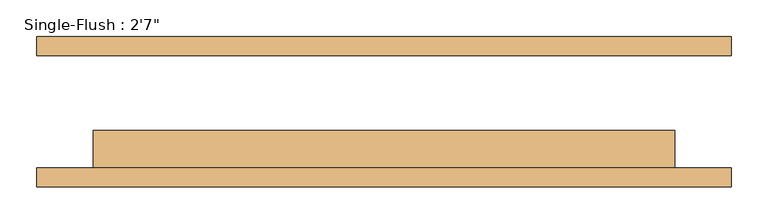
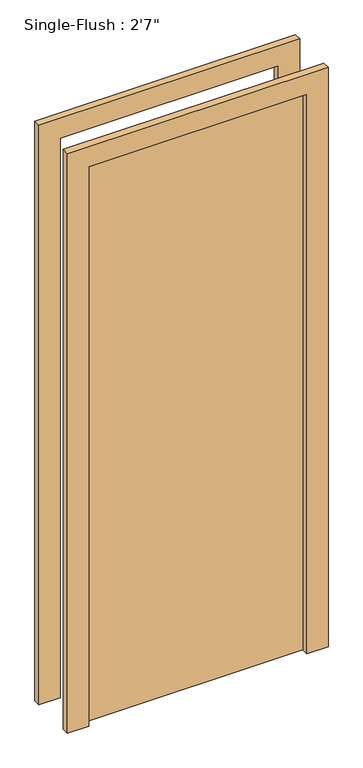
"""IFC4 building model written with IfcOpenShell, lengths in millimetres: door geometry."""

from ifc_helpers import new_model, si_unit, frame, origin, origin_with_axes, place, context, project, spatial, polyline, outline, extrude, source, transform, mapped, element, save


def door_dc34e247(model_context):
    return source(origin(), model_context, "Body", "SweptSolid", [
        extrude(outline(polyline([(2209.8, -469.9), (0.0, -469.9), (0.0, -393.7), (2133.6, -393.7), (2133.6, 393.7), (0.0, 393.7), (0.0, 469.9), (2209.8, 469.9), (2209.8, -469.9)])), frame((0.0, -101.6, 0.0), z_axis=(0.0, 1.0, 0.0), x_axis=(0.0, 0.0, 1.0)), (0.0, 0.0, 1.0), 25.4),
        extrude(outline(polyline([(2209.8, 469.9), (2209.8, -469.9), (0.0, -469.9), (0.0, -393.7), (2133.6, -393.7), (2133.6, 393.7), (0.0, 393.7), (0.0, 469.9), (2209.8, 469.9)])), frame((0.0, 76.2, 0.0), z_axis=(0.0, 1.0, 0.0), x_axis=(0.0, 0.0, 1.0)), (0.0, 0.0, 1.0), 25.4),
        extrude(outline(polyline([(393.7, -25.4), (393.7, -76.2), (-393.7, -76.2), (-393.7, -25.4), (393.7, -25.4)])), origin_with_axes(), (0.0, 0.0, 1.0), 2133.6),
    ])


if __name__ == "__main__":
    model = new_model("IFC4")
    model_context = context("Model", 3, world=origin())
    ifc_project = project(units=[si_unit("LENGTHUNIT", "METRE", prefix="MILLI")], contexts=[model_context])
    site = spatial("IfcSite", under=ifc_project)
    building = spatial("IfcBuilding", under=site)
    placement = place(None, origin())
    door_shape = door_dc34e247(model_context)
    element("IfcDoor", 1, ObjectType="Single-Flush : 2'7\"", at=placement, inside=building, context=model_context, shape_type="MappedRepresentation", body=[
        mapped(door_shape, transform((0.0, 0.0, 0.0), x_axis=(1.0, 0.0, 0.0), y_axis=(0.0, 1.0, 0.0), z_axis=(0.0, 0.0, 1.0))),
    ])
    save(model, "model.ifc")

# Revit data of these elements
# Type "Single-Flush : 2'7\""
#   Type Mark = "8"
#   Construction Type Id = "MDOOR"
#   Assembly Code = "C1020"
#   Analytic Construction = "Metal"
#   Thickness = 0' - 2"
#   Heat Transfer Coefficient (U) = 0.651978 BTU/(h·ft²·°F)
#   Height = 7' - 0"
#   Trim Projection Ext = 0' - 1"
#   Trim Projection Int = 0' - 1"
#   Trim Width = 0' - 3"
#   Width = 2' - 7"
#   Define Thermal Properties by = 1
#   Door Material = Door - Panel
#   Frame Material = Door - Frame
#   Visual Light Transmittance = 0
#   Solar Heat Gain Coefficient = 0
#   Function = (empty or 0)
#   Wall Closure = (empty or 0)
# Element 1 (IfcDoor, "Single-Flush : 2'7\"")
#   Materials on its faces: "Door - Frame", "Door - Panel"
# Materials
#   "Door - Panel": class "Wood", colour RGB 210 159 95, transparency 0, Cost = 0
#   "Door - Frame": colour RGB 118 70 51, transparency 0, Cost = 0
